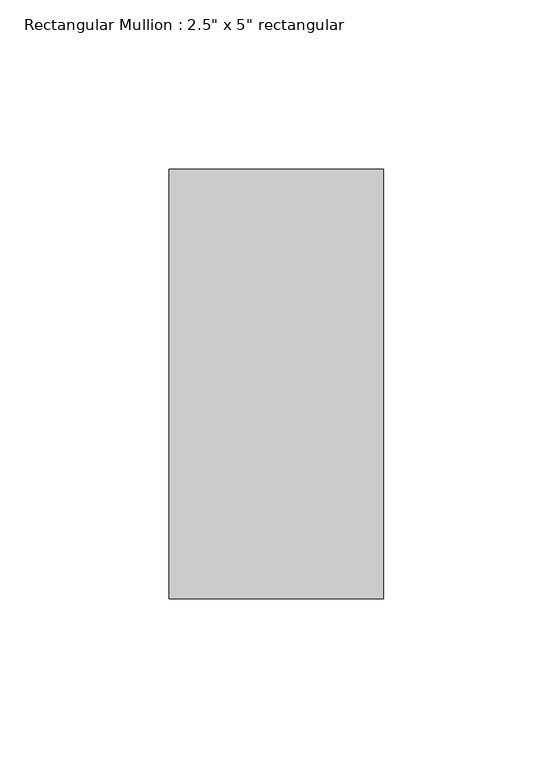
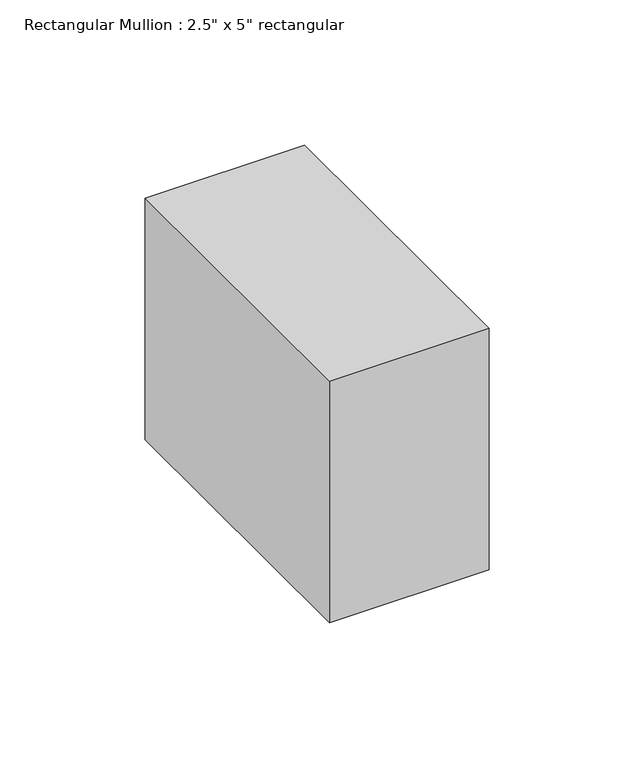
"""IFC4 building model written with IfcOpenShell, lengths in millimetres: member geometry."""

from ifc_helpers import new_model, si_unit, frame, origin, place, context, project, spatial, polyline, outline, extrude, source, transform, mapped, element, save


def member_fb13da3b(model_context):
    return source(origin(), model_context, "Body", "SweptSolid", [
        extrude(outline(polyline([(0.0, 63.5), (0.0, -63.5), (-63.5, -63.5), (-63.5, 63.5), (0.0, 63.5)])), frame((0.0, 0.0, -101.6), z_axis=(0.0, 0.0, 1.0), x_axis=(1.0, 0.0, 0.0)), (0.0, 0.0, 1.0), 101.6),
    ])


if __name__ == "__main__":
    model = new_model("IFC4")
    model_context = context("Model", 3, world=origin())
    ifc_project = project(units=[si_unit("LENGTHUNIT", "METRE", prefix="MILLI")], contexts=[model_context])
    site = spatial("IfcSite", under=ifc_project)
    building = spatial("IfcBuilding", under=site)
    placement = place(None, origin())
    member_shape = member_fb13da3b(model_context)
    element("IfcMember", 1, ObjectType="Rectangular Mullion : 2.5\" x 5\" rectangular", at=placement, inside=building, context=model_context, shape_type="MappedRepresentation", body=[
        mapped(member_shape, transform((0.0, 0.0, 0.0), x_axis=(1.0, 0.0, 0.0), y_axis=(0.0, 1.0, 0.0), z_axis=(0.0, 0.0, 1.0))),
    ])
    save(model, "model.ifc")

# Revit data of these elements
# Type "Rectangular Mullion : 2.5\" x 5\" rectangular"
#   built-in parameter 1007304 = 0.416667 (stored number, unit not read)
#   built-in parameter 1007301 = 0.104167 (stored number, unit not read)
#   built-in parameter 1007300 = 0.104167 (stored number, unit not read)
# Element 1 (IfcMember, "Rectangular Mullion : 2.5\" x 5\" rectangular")
#   Materials on its faces: "Aluminum"
# Materials
#   "Aluminum": class "Metal", colour RGB 247 247 247, transparency 0, Description = "Aluminum 6061", Cost = 0
